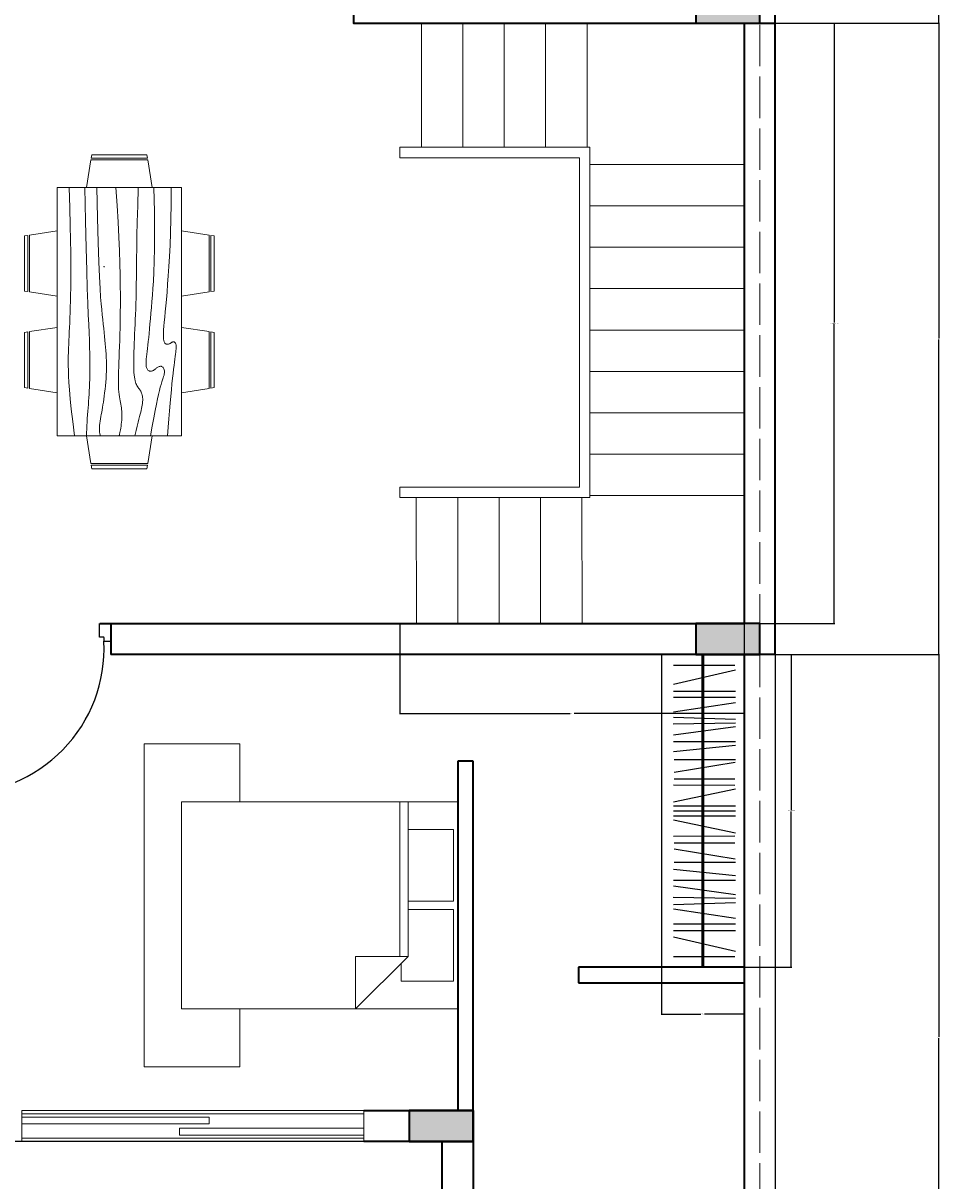
# Model space of a CAD drawing. Units: inches. Extents: x 2711 to 4246, y 540 to 1583.
# Tile 3 of 7: x 3086 to 3351, y 894 to 1230. Entities that reach past the tile are written whole.
import ezdxf

# ---------------------------------------------------------------- set-up
doc = ezdxf.new("R2010")
doc.units = ezdxf.units.IN
doc.linetypes.add('ACAD_ISO02W100', pattern=[15, 12, -3])
for name, color, linetype, lineweight in [('A-ANNO-DIMS', 2, 'Continuous', 18), ('A-COLS', 210, 'Continuous', 35), ('A-COLS-PATT', 6, 'Continuous', 13), ('A-FLOR-CASE', 30, 'Continuous', 18), ('A-FLOR-STRS', 4, 'Continuous', 18), ('A-GLAZ', 4, 'Continuous', 18), ('A-WALL', 1, 'Continuous', 35), ('C-PROP-HIDN', 7, 'ACAD_ISO02W100', 13), ('C-PROP-WALL', 7, 'Continuous', 25), ('DOOR', 32, 'Continuous', 25), ('FURN', 30, 'Continuous', 18)]:
    doc.layers.add(name, color=color, linetype=linetype, lineweight=lineweight)
doc.layers.add('DECOR', color=30, linetype='Continuous')
doc.styles.get("Standard").update_dxf_attribs({"font": 'arial.ttf'})
doc.dimstyles.get("Standard").update_dxf_attribs({"dimtxt": 0.18, "dimasz": 0.18, "dimexe": 0.18, "dimexo": 0.0625, "dimgap": 0.09, "dimtad": 0, "dimtih": 1, "dimtoh": 1, "dimdec": 4, "dimzin": 0, "dimdsep": 46, "dimtxsty": 'Standard', "dimcen": 0.09, "dimadec": 0, "dimazin": 0, "dimtfac": 1, "dimtdec": 4, "dimtofl": 0, "dimtmove": 0, "dimatfit": 3, "dimfxl": 1, "dimtolj": 1, "dimtzin": 0, "dimarcsym": 0})

# ---------------------------------------------------------------- blocks, each defined once
blk = doc.blocks.new('DOORS')
at = {"layer": 'DOOR'}
for p, q in [((-0.63, -0.36), (-0.63, -5.61)), ((2.62, -4.36), (2.62, -0.36)), ((44.12, -4.36), (44.12, -0.36)), ((47.37, -0.36), (47.37, -5.61)), ((-0.63, -5.61), (1.37, -5.61)), ((1.37, -5.61), (1.37, -4.36)), ((1.37, -4.36), (2.62, -4.36)), ((1.37, -5.61), (1.37, -49.61)), ((2.37, -49.61), (2.37, -4.36)), ((45.37, -4.36), (44.12, -4.36)), ((47.37, -5.61), (45.37, -5.61)), ((1.37, -49.61), (2.37, -49.61))]:
    blk.add_line(p, q, dxfattribs=at)
for centre, radius, start, end in [((3.41, -7.61), 42.01, 268.5852, 2.7319), ((38.76, -4.99), 6.64, 354.6023, 5.3977)]:
    blk.add_arc(centre, radius, start, end, dxfattribs=at)
blk = doc.blocks.new('WARDROBE')
at = {"layer": 'DECOR'}
for p, q in [((24, 0), (0, 0)), ((0, 0), (0, -90.69)), ((11.75, 0), (11.75, -90.69)), ((11.78, 0), (11.78, -90.69)), ((11.8, 0), (11.8, -90.69)), ((11.83, 0), (11.83, -90.69)), ((11.85, 0), (11.85, -90.69)), ((11.88, 0), (11.88, -90.69)), ((11.92, 0), (11.92, -90.69)), ((11.95, 0), (11.95, -90.69)), ((11.97, 0), (11.97, -90.69)), ((12, 0), (12, -90.69)), ((12.03, 0), (12.03, -90.69)), ((12.06, 0), (12.06, -90.69)), ((12.1, 0), (12.1, -90.69)), ((12.14, 0), (12.14, -90.69)), ((12.17, 0), (12.17, -90.69)), ((12.2, 0), (12.2, -90.69)), ((12.22, 0), (12.22, -90.69)), ((12.25, 0), (12.25, -90.69)), ((12.25, 0), (12.25, -90.69)), ((24, -90.69), (24, 0)), ((3.53, -3.09), (21.27, -3.09)), ((21.48, -4.58), (3.53, -8.75)), ((3.53, -10.65), (21.48, -10.65)), ((21.48, -12.45), (3.53, -12.45)), ((21.48, -14.08), (3.53, -16.79)), ((21.48, -19.96), (3.47, -20.22)), ((3.53, -18.23), (21.48, -18.75)), ((21.49, -21.01), (3.52, -23.46)), ((3.52, -25.25), (21.49, -25.25)), ((21.49, -26.46), (3.52, -28.29)), ((3.74, -30.44), (21.49, -30.44)), ((21.36, -31.31), (3.74, -34.21)), ((3.74, -36.1), (21.29, -36.1)), ((21.29, -37.99), (3.52, -37.93)), ((3.52, -42.71), (21.49, -38.99)), ((3.52, -43.88), (21.49, -43.88)), ((3.52, -45.34), (21.49, -45.34)), ((3.52, -46.81), (21.49, -46.81)), ((3.52, -47.98), (21.49, -51.69)), ((21.29, -52.7), (3.52, -52.76)), ((3.74, -54.59), (21.29, -54.59)), ((21.36, -59.38), (3.74, -56.48)), ((3.74, -60.25), (21.49, -60.25)), ((21.49, -64.22), (3.52, -62.4)), ((3.52, -65.43), (21.49, -65.43)), ((21.48, -70.73), (3.47, -70.47)), ((21.49, -69.68), (3.52, -67.23)), ((3.53, -72.46), (21.48, -71.94)), ((21.48, -76.61), (3.53, -73.9)), ((21.48, -78.24), (3.53, -78.24)), ((3.53, -80.04), (21.48, -80.04)), ((21.48, -86.1), (3.53, -81.94)), ((3.53, -87.59), (21.27, -87.59)), ((0, -90.69), (24, -90.69))]:
    blk.add_line(p, q, dxfattribs=at)
blk = doc.blocks.new('Bed - Queen')
for p, q in [((0, -80.00003), (0, 0)), ((0, 0), (59.99999, 0)), ((59.99999, 0), (59.99999, -80.00003)), ((7.99999, -1.2), (28.79998, -1.2)), ((7.99999, -14.4), (7.99999, -1.2)), ((28.79998, -1.2), (28.79998, -14.4)), ((31.19999, -1.2), (51.99999, -1.2)), ((31.19999, -14.4), (31.19999, -1.2)), ((51.99999, -1.2), (51.99999, -16.4)), ((0, -14.4), (44.8, -14.4)), ((59.99999, -29.6), (44.8, -14.4)), ((44.8, -14.4), (44.8, -29.6)), ((51.99999, -16.4), (46.79936, -16.4)), ((44.8, -16.8), (0, -16.8)), ((44.8, -29.6), (59.99999, -29.6)), ((59.99999, -80.00003), (0, -80.00003))]:
    blk.add_line(p, q)
blk = doc.blocks.new('Dining Set - 36 x 72 in.')
for p, q in [((-22, 27.5), (-22.1562, 26.50042)), ((-22, 27.5), (-6, 27.5)), ((-5.8437, 26.49966), (-6, 27.5)), ((6, 27.5), (5.8438, 26.50042)), ((6, 27.5), (22, 27.5)), ((22.1563, 26.49966), (22, 27.5)), ((-22.2343, 26.00059), (-23.4847, 17.99762)), ((-22.2304, 26), (-5.7608, 26)), ((-5.8416, 26.5), (-22.1534, 26.5)), ((-4.5152, 17.99762), (-5.7655, 25.99926)), ((5.7657, 26.00059), (4.5153, 17.99762)), ((5.7696, 26), (22.2392, 26)), ((22.1584, 26.5), (5.8466, 26.5)), ((23.4848, 17.99762), (22.2345, 25.99926)), ((36, 18), (-36, 18)), ((-36, 18), (-36, -18)), ((36, -18), (36, 18)), ((-45.5, 8), (-44.5004, 8.15617)), ((-45.5, 8), (-45.5, -8)), ((-44.5, -8.15843), (-44.5, 8.15338)), ((-44.0006, 8.23428), (-35.9976, 9.48474)), ((-44, 8.23041), (-44, -8.23915)), ((44.0006, 8.23428), (35.9976, 9.48474)), ((44, 8.23041), (44, -8.23915)), ((44.5, -8.15843), (44.5, 8.15338)), ((45.5, 8), (44.5005, 8.15617)), ((45.5, 8), (45.5, -8)), ((-44.4997, -8.15631), (-45.5, -8)), ((-35.9976, -9.48476), (-43.9993, -8.2345)), ((35.9976, -9.48476), (43.9993, -8.2345)), ((44.4997, -8.15631), (45.5, -8)), ((-36, -18), (36, -18)), ((-22.2343, -26.0006), (-23.4847, -17.99762)), ((-4.5152, -17.99762), (-5.7655, -25.99928)), ((5.7657, -26.0006), (4.5153, -17.99762)), ((23.4848, -17.99762), (22.2345, -25.99928)), ((-22.2304, -26), (-5.7608, -26)), ((-22, -27.5), (-22.1562, -26.50044)), ((-5.8416, -26.5), (-22.1534, -26.5)), ((-5.8437, -26.49967), (-6, -27.5)), ((5.7696, -26), (22.2392, -26)), ((6, -27.5), (5.8438, -26.50044)), ((22.1584, -26.5), (5.8466, -26.5)), ((22.1563, -26.49967), (22, -27.5)), ((-22, -27.5), (-6, -27.5)), ((6, -27.5), (22, -27.5))]:
    blk.add_line(p, q)
for points in [[(-36, 15), (-31.1772, 14.97754), (-26.8079, 14.91406), (-22.8538, 14.81543), (-19.276, 14.6875), (-16.0362, 14.53613), (-13.0957, 14.36718), (-10.4159, 14.18652), (-7.9583, 14), (-5.6904, 13.81315), (-3.6035, 13.63021), (-1.6954, 13.45508), (0.0365, 13.29166), (1.5945, 13.14388), (2.9811, 13.01562), (4.1988, 12.9108), (5.25, 12.83333), (6.1393, 12.78613), (6.8802, 12.76823), (7.4883, 12.77767), (7.9792, 12.8125), (8.3685, 12.87077), (8.6719, 12.95052), (8.9049, 13.0498), (9.0833, 13.16666), (9.2205, 13.29899), (9.3216, 13.44401), (9.3895, 13.59879), (9.4271, 13.76041), (9.4373, 13.92594), (9.4232, 14.09245), (9.3875, 14.257), (9.3333, 14.41666), (9.2638, 14.56917), (9.1836, 14.71484), (9.0975, 14.85465), (9.0104, 14.98958), (8.9272, 15.1206), (8.8529, 15.2487), (8.7922, 15.37483), (8.75, 15.5), (8.7305, 15.62467), (8.7344, 15.74739), (8.7617, 15.86621), (8.8125, 15.97916), (8.8867, 16.08431), (8.9844, 16.17968), (9.1055, 16.26334), (9.25, 16.33333), (9.4189, 16.38802), (9.6172, 16.42708), (9.8506, 16.45052), (10.125, 16.45833), (10.4463, 16.45052), (10.8203, 16.42708), (11.2529, 16.38802), (11.75, 16.33333), (12.3184, 16.26318), (12.9694, 16.17838), (13.7151, 16.07991), (14.5677, 15.96875), (15.5395, 15.84586), (16.6426, 15.71224), (17.8893, 15.56884), (19.2917, 15.41666), (20.859, 15.25667), (22.5879, 15.08984), (24.4721, 14.91715), (26.5052, 14.73958), (28.6809, 14.5581), (30.9929, 14.3737), (33.4347, 14.18733), (36, 14)], [(-36, 10), (-28.9766, 10.14274), (-23.1725, 10.20442), (-18.4241, 10.19775), (-14.5677, 10.13541), (-11.4399, 10.03011), (-8.877, 9.89453), (-6.7154, 9.74137), (-4.7917, 9.58333), (-2.9698, 9.43082), (-1.2246, 9.28515), (0.4415, 9.14534), (2.026, 9.01041), (3.5266, 8.87939), (4.9408, 8.7513), (6.266, 8.62516), (7.5, 8.5), (8.6411, 8.37549), (9.6914, 8.2539), (10.6538, 8.13818), (11.5312, 8.03125), (12.3267, 7.93603), (13.043, 7.85547), (13.6831, 7.79248), (14.25, 7.75), (14.7471, 7.7303), (15.1797, 7.73307), (15.5537, 7.75732), (15.875, 7.80208), (16.1494, 7.86637), (16.3828, 7.94922), (16.5811, 8.04964), (16.75, 8.16666), (16.8944, 8.29915), (17.0143, 8.44531), (17.1089, 8.60319), (17.1771, 8.77083), (17.218, 8.94629), (17.2305, 9.1276), (17.2137, 9.31282), (17.1667, 9.5), (17.0895, 9.6875), (16.987, 9.875), (16.8649, 10.0625), (16.7292, 10.25), (16.5856, 10.4375), (16.4401, 10.625), (16.2985, 10.8125), (16.1667, 11), (16.05, 11.18733), (15.9518, 11.3737), (15.8752, 11.5581), (15.8229, 11.73958), (15.798, 11.91715), (15.8034, 12.08984), (15.842, 12.25667), (15.9167, 12.41666), (16.0295, 12.56836), (16.1784, 12.70833), (16.3605, 12.83268), (16.5729, 12.9375), (16.8127, 13.01888), (17.0768, 13.07291), (17.3625, 13.0957), (17.6667, 13.08333), (17.9894, 13.03312), (18.3418, 12.94726), (18.7382, 12.82918), (19.1927, 12.68229), (19.7195, 12.51001), (20.3327, 12.31575), (21.0465, 12.10294), (21.875, 11.875), (22.8357, 11.63354), (23.959, 11.37304), (25.2786, 11.08618), (26.8282, 10.76562), (28.6414, 10.40405), (30.752, 9.99414), (33.1936, 9.52856), (36, 9)], [(-36, 5.5), (-30.7157, 5.3348), (-26.069, 5.20963), (-21.9946, 5.11767), (-18.4271, 5.05208), (-15.3009, 5.00602), (-12.5508, 4.97265), (-10.1112, 4.94515), (-7.9167, 4.91666), (-5.909, 4.88167), (-4.0586, 4.83984), (-2.3429, 4.79215), (-0.7396, 4.73958), (0.7739, 4.6831), (2.22, 4.6237), (3.6213, 4.56233), (5, 4.5), (6.373, 4.43782), (7.7344, 4.3776), (9.0723, 4.32129), (10.375, 4.27083), (11.6309, 4.22819), (12.8281, 4.19531), (13.9551, 4.17415), (15, 4.16666), (15.954, 4.17448), (16.819, 4.19791), (17.6001, 4.23698), (18.3021, 4.29166), (18.9299, 4.36198), (19.4883, 4.44791), (19.9823, 4.54948), (20.4167, 4.66666), (20.7969, 4.79899), (21.1302, 4.94401), (21.4245, 5.09879), (21.6875, 5.26041), (21.9271, 5.42594), (22.1511, 5.59245), (22.3672, 5.757), (22.5834, 5.91666), (22.8065, 6.06868), (23.0404, 6.21093), (23.2879, 6.34147), (23.5521, 6.45833), (23.8358, 6.55957), (24.142, 6.64323), (24.4735, 6.70735), (24.8334, 6.75), (25.2235, 6.76969), (25.642, 6.76692), (26.0858, 6.74267), (26.5521, 6.69791), (27.0379, 6.63362), (27.5404, 6.55078), (28.0565, 6.45036), (28.5834, 6.33333), (29.1242, 6.19987), (29.7071, 6.04687), (30.3661, 5.87044), (31.1354, 5.66666), (32.0493, 5.43164), (33.142, 5.16146), (34.4475, 4.85221), (36, 4.5)], [(-36, -1), (-30.7915, -0.6591), (-26.0195, -0.38216), (-21.6519, -0.16284), (-17.6563, 0.00521), (-14.0005, 0.12833), (-10.6523, 0.21289), (-7.5796, 0.26522), (-4.75, 0.29166), (-2.134, 0.29793), (0.2878, 0.28711), (2.5317, 0.26163), (4.6146, 0.22396), (6.5529, 0.17651), (8.3633, 0.12174), (10.0623, 0.06209), (11.6667, 0), (13.1899, -0.06201), (14.6341, -0.1211), (15.9982, -0.17432), (17.2813, -0.21875), (18.4823, -0.25147), (19.6003, -0.26953), (20.6343, -0.27002), (21.5834, -0.25), (22.4481, -0.20768), (23.2357, -0.14584), (23.9549, -0.06836), (24.6146, 0.02083), (25.2235, 0.11784), (25.7904, 0.21875), (26.3241, 0.31966), (26.8334, 0.41666), (27.3265, 0.50618), (27.8099, 0.58593), (28.2894, 0.65397), (28.7709, 0.70833), (29.2601, 0.74707), (29.763, 0.76823), (30.2855, 0.76985), (30.8334, 0.75), (31.4088, 0.70784), (31.9994, 0.64713), (32.589, 0.57275), (33.1615, 0.48958), (33.7008, 0.4025), (34.1908, 0.3164), (34.6153, 0.23616), (34.9584, 0.16666), (35.2099, 0.11165), (35.3848, 0.07031), (35.504, 0.04069), (35.5886, 0.02083), (35.6594, 0.00879), (35.7377, 0.0026), (35.8442, 0.00032), (36, 0)], [(-36, -6.5), (-27.1843, -6.31267), (-20.084, -6.1263), (-14.469, -5.9419), (-10.1094, -5.76042), (-6.7752, -5.58285), (-4.2363, -5.41016), (-2.2629, -5.24333), (-0.625, -5.08334), (0.8708, -4.93099), (2.2715, -4.78646), (3.5872, -4.64974), (4.8281, -4.52084), (6.0046, -4.39974), (7.127, -4.28646), (8.2053, -4.18099), (9.25, -4.08334), (10.2705, -3.99382), (11.2734, -3.91407), (12.2647, -3.84603), (13.25, -3.79167), (14.2354, -3.75293), (15.2266, -3.73177), (16.2295, -3.73015), (17.25, -3.75), (18.2912, -3.79248), (19.3451, -3.85547), (20.4009, -3.93604), (21.4479, -4.03125), (22.4754, -4.13819), (23.4727, -4.25391), (24.4289, -4.37549), (25.3334, -4.5), (26.1785, -4.62492), (26.9694, -4.74935), (27.7145, -4.87281), (28.4219, -4.99479), (29.1, -5.11483), (29.7572, -5.23242), (30.4016, -5.34709), (31.0417, -5.45834), (31.6837, -5.56437), (32.3262, -5.65821), (32.9658, -5.73153), (33.599, -5.77604), (34.2224, -5.78345), (34.8327, -5.74545), (35.4264, -5.65373), (36, -5.5)], [(-36, -10), (-26.4022, -9.81299), (-18.4675, -9.62891), (-11.9839, -9.45069), (-6.7396, -9.28125), (-2.5226, -9.12354), (0.8789, -8.98047), (3.6769, -8.85498), (6.0833, -8.75), (8.2767, -8.66765), (10.3021, -8.60677), (12.1712, -8.56543), (13.8958, -8.54167), (15.4876, -8.53353), (16.9583, -8.53907), (18.3197, -8.55632), (19.5834, -8.58334), (20.7616, -8.61841), (21.8685, -8.66081), (22.9188, -8.71004), (23.9271, -8.76563), (24.9081, -8.82707), (25.8763, -8.89388), (26.8465, -8.96558), (27.8334, -9.04167), (28.8474, -9.12118), (29.8828, -9.20117), (30.93, -9.27824), (31.9792, -9.34896), (33.0205, -9.40991), (34.0443, -9.45768), (35.0407, -9.48885), (36, -9.5)], [(-36, -14.5), (-30.0881, -14.33513), (-25.0332, -14.21224), (-20.7312, -14.12647), (-17.0781, -14.07292), (-13.97, -14.04671), (-11.3027, -14.04297), (-8.9724, -14.05681), (-6.875, -14.08334), (-4.9224, -14.11833), (-3.0905, -14.16016), (-1.3709, -14.20785), (0.2448, -14.26042), (1.7647, -14.3169), (3.1973, -14.3763), (4.5507, -14.43767), (5.8333, -14.5), (7.0554, -14.5621), (8.235, -14.62175), (9.3922, -14.67652), (10.5469, -14.72396), (11.7192, -14.76164), (12.929, -14.78711), (14.1965, -14.79794), (15.5417, -14.79167), (16.9933, -14.76424), (18.6152, -14.70508), (20.4804, -14.60197), (22.6615, -14.44271), (25.2312, -14.21509), (28.2624, -13.9069), (31.8277, -13.50594), (36, -13)]]:
    blk.add_lwpolyline(points)
blk = doc.blocks.new('STAIR-RETURN')
for p, q in [((6.2, 174.01), (6.2, 138.01)), ((18.2, 174.01), (18.2, 138.01)), ((30.2, 174.01), (30.2, 138.01)), ((42.2, 174.01), (42.2, 138.01)), ((54.2, 174.01), (54.2, 138.01)), ((55.04, 138.01), (0, 138.01)), ((0, 138.01), (0, 135.01)), ((55.04, 133.05), (55.04, 138.01)), ((52.04, 135.01), (0, 135.01)), ((52.04, 39.5), (52.04, 135.01)), ((99.72, 133.05), (55.04, 133.05)), ((55.04, 37.05), (55.04, 133.05)), ((99.72, 121.05), (55.04, 121.05)), ((99.72, 109.05), (55.04, 109.05)), ((99.72, 97.05), (55.04, 97.05)), ((99.72, 85.05), (55.04, 85.05)), ((99.72, 73.05), (55.04, 73.05)), ((99.72, 61.05), (55.04, 61.05)), ((99.72, 49.05), (55.04, 49.05)), ((0, 36.5), (0, 39.5)), ((0, 39.5), (52.04, 39.5)), ((99.72, 37.05), (55.04, 37.05)), ((55.04, 36.5), (55.04, 37.05)), ((0, 36.5), (52.73, 36.5)), ((4.73, 36.5), (4.74, 0)), ((16.73, 36.5), (16.74, 0)), ((28.73, 36.5), (28.74, 0)), ((40.73, 36.5), (40.74, 0)), ((52.73, 36.5), (52.74, 0)), ((52.73, 36.5), (55.04, 36.5))]:
    blk.add_line(p, q)
blk = doc.blocks.new('WIN-SLIDER-W03')
for p, q in [((0, 9), (0, 0)), ((99.07, 9), (0, 9)), ((0, 8.03), (99.07, 8.03)), ((0, 7.05), (54.2, 7.05)), ((54.2, 7.05), (54.2, 5.05)), ((99.07, 9), (99.07, 0)), ((54.2, 5.05), (0, 5.05)), ((45.64, 1.82), (45.64, 3.82)), ((45.64, 3.82), (99.07, 3.82)), ((0, 0.97), (99.07, 0.97)), ((99.07, 1.82), (45.64, 1.82)), ((0, 0), (99.07, 0))]:
    blk.add_line(p, q)
blk = doc.blocks.new('BED-BASE-QUEEN')
for p, q in [((27.64, 93.59), (0, 93.59)), ((0, 93.59), (0, 46.79)), ((27.64, 76.79), (27.64, 93.59)), ((0, 0), (0, 46.79)), ((27.64, 16.79), (27.64, 0)), ((27.64, 0), (0, 0))]:
    blk.add_line(p, q)
blk = doc.blocks.new('*D74')
at = {"layer": 'A-ANNO-DIMS', "color": 0, "lineweight": -2, "transparency": 16777216}
for p, q in [((3294.56, 1046.95), (3308.28, 1046.95)), ((3308.1, 1046.77), (3308.1, 1001.79)), ((3308.1, 956.44), (3308.1, 1001.42)), ((3294.56, 956.26), (3308.28, 956.26))]:
    blk.add_line(p, q, dxfattribs=at)
at = {"layer": 'A-ANNO-DIMS', "color": 0, "transparency": 16777216}
for points in [[(3308.07, 1046.77), (3308.13, 1046.77), (3308.1, 1046.95)], [(3308.07, 956.44), (3308.13, 956.44), (3308.1, 956.26)]]:
    blk.add_solid(points, dxfattribs=at)
at = {"layer": 'Defpoints', "color": 0, "transparency": 16777216}
for p in [(3294.5, 1046.95), (3308.1, 1046.95), (3294.5, 956.26)]:
    blk.add_point(p, dxfattribs=at)
at = {"layer": 'A-ANNO-DIMS', "color": 0, "transparency": 16777216, "insert": (3308.1, 1001.61), "char_height": 0.18, "attachment_point": 5}
blk.add_mtext('\\A1;WARDROBE 91 TYP.', dxfattribs=at)
blk = doc.blocks.new('*D75')
at = {"layer": 'A-ANNO-DIMS', "color": 0, "lineweight": -2, "transparency": 16777216}
for p, q in [((3270.5, 956.2), (3270.5, 942.48)), ((3294.5, 956.2), (3294.5, 942.48)), ((3270.68, 942.66), (3281.97, 942.66)), ((3294.32, 942.66), (3283.03, 942.66))]:
    blk.add_line(p, q, dxfattribs=at)
at = {"layer": 'A-ANNO-DIMS', "color": 0, "transparency": 16777216}
for points in [[(3270.68, 942.69), (3270.68, 942.63), (3270.5, 942.66)], [(3294.32, 942.69), (3294.32, 942.63), (3294.5, 942.66)]]:
    blk.add_solid(points, dxfattribs=at)
at = {"layer": 'Defpoints', "color": 0, "transparency": 16777216}
for p in [(3270.5, 956.26), (3294.5, 956.26), (3294.5, 942.66)]:
    blk.add_point(p, dxfattribs=at)
at = {"layer": 'A-ANNO-DIMS', "color": 0, "transparency": 16777216, "insert": (3282.5, 942.66), "char_height": 0.18, "attachment_point": 5}
blk.add_mtext('\\A1;24 TYP.', dxfattribs=at)
blk = doc.blocks.new('*D82')
at = {"layer": 'A-ANNO-DIMS', "color": 0, "lineweight": -2, "transparency": 16777216}
for p, q in [((3294.56, 1229.95), (3320.78, 1229.95)), ((3320.6, 1229.77), (3320.6, 1143.13)), ((3320.6, 1056.12), (3320.6, 1142.76)), ((3294.56, 1055.94), (3320.78, 1055.94))]:
    blk.add_line(p, q, dxfattribs=at)
at = {"layer": 'A-ANNO-DIMS', "color": 0, "transparency": 16777216}
for points in [[(3320.57, 1229.77), (3320.63, 1229.77), (3320.6, 1229.95)], [(3320.57, 1056.12), (3320.63, 1056.12), (3320.6, 1055.94)]]:
    blk.add_solid(points, dxfattribs=at)
at = {"layer": 'Defpoints', "color": 0, "transparency": 16777216}
for p in [(3294.5, 1229.95), (3320.6, 1229.95), (3294.5, 1055.94)]:
    blk.add_point(p, dxfattribs=at)
at = {"layer": 'A-ANNO-DIMS', "color": 0, "transparency": 16777216, "insert": (3320.6, 1142.95), "char_height": 0.18, "attachment_point": 5}
blk.add_mtext('\\A1;RETURN STAIR 174 TYP.', dxfattribs=at)
blk = doc.blocks.new('*D83')
at = {"layer": 'A-ANNO-DIMS', "color": 0, "lineweight": -2, "transparency": 16777216}
for p, q in [((3194.77, 1055.88), (3194.77, 1029.66)), ((3294.5, 1055.88), (3294.5, 1029.66)), ((3194.95, 1029.84), (3244.05, 1029.84)), ((3294.32, 1029.84), (3245.22, 1029.84))]:
    blk.add_line(p, q, dxfattribs=at)
at = {"layer": 'A-ANNO-DIMS', "color": 0, "transparency": 16777216}
for points in [[(3194.95, 1029.87), (3194.95, 1029.81), (3194.77, 1029.84)], [(3294.32, 1029.87), (3294.32, 1029.81), (3294.5, 1029.84)]]:
    blk.add_solid(points, dxfattribs=at)
at = {"layer": 'Defpoints', "color": 0, "transparency": 16777216}
for p in [(3194.77, 1055.94), (3294.5, 1055.94), (3294.5, 1029.84)]:
    blk.add_point(p, dxfattribs=at)
at = {"layer": 'A-ANNO-DIMS', "color": 0, "transparency": 16777216, "insert": (3244.63, 1029.84), "char_height": 0.18, "attachment_point": 5}
blk.add_mtext('\\A1;100 TYP.', dxfattribs=at)
blk = doc.blocks.new('*D99')
at = {"layer": 'A-ANNO-DIMS', "color": 0, "lineweight": -2, "transparency": 16777216}
for p, q in [((3299.06, 1046.94), (3351.05, 1046.94)), ((3350.87, 1046.76), (3350.87, 936.03)), ((3350.87, 824.93), (3350.87, 935.67)), ((3299.06, 824.75), (3351.05, 824.75))]:
    blk.add_line(p, q, dxfattribs=at)
at = {"layer": 'A-ANNO-DIMS', "color": 0, "transparency": 16777216}
for points in [[(3350.84, 1046.76), (3350.9, 1046.76), (3350.87, 1046.94)], [(3350.84, 824.93), (3350.9, 824.93), (3350.87, 824.75)]]:
    blk.add_solid(points, dxfattribs=at)
at = {"layer": 'Defpoints', "color": 0, "transparency": 16777216}
for p in [(3299, 1046.94), (3350.87, 1046.94), (3299, 824.75)]:
    blk.add_point(p, dxfattribs=at)
at = {"layer": 'A-ANNO-DIMS', "color": 0, "transparency": 16777216, "insert": (3350.87, 935.85), "char_height": 0.18, "attachment_point": 5}
blk.add_mtext('\\A1;222.2', dxfattribs=at)
blk = doc.blocks.new('*D100')
at = {"layer": 'A-ANNO-DIMS', "color": 0, "lineweight": -2, "transparency": 16777216}
for p, q in [((3299.06, 1229.95), (3351.05, 1229.95)), ((3350.87, 1229.77), (3350.87, 1138.63)), ((3350.87, 1047.12), (3350.87, 1138.26)), ((3299.06, 1046.94), (3351.05, 1046.94))]:
    blk.add_line(p, q, dxfattribs=at)
at = {"layer": 'A-ANNO-DIMS', "color": 0, "transparency": 16777216}
for points in [[(3350.84, 1229.77), (3350.9, 1229.77), (3350.87, 1229.95)], [(3350.84, 1047.12), (3350.9, 1047.12), (3350.87, 1046.94)]]:
    blk.add_solid(points, dxfattribs=at)
at = {"layer": 'Defpoints', "color": 0, "transparency": 16777216}
for p in [(3299, 1229.95), (3350.87, 1229.95), (3299, 1046.94)]:
    blk.add_point(p, dxfattribs=at)
at = {"layer": 'A-ANNO-DIMS', "color": 0, "transparency": 16777216, "insert": (3350.87, 1138.45), "char_height": 0.18, "attachment_point": 5}
blk.add_mtext('\\A1;183', dxfattribs=at)
blk = doc.blocks.new('*D101')
at = {"layer": 'A-ANNO-DIMS', "color": 0, "lineweight": -2, "transparency": 16777216}
for p, q in [((3209.06, 1289.95), (3351.05, 1289.95)), ((3350.87, 1289.77), (3350.87, 1260.13)), ((3350.87, 1230.13), (3350.87, 1259.77)), ((3299.06, 1229.95), (3351.05, 1229.95))]:
    blk.add_line(p, q, dxfattribs=at)
at = {"layer": 'A-ANNO-DIMS', "color": 0, "transparency": 16777216}
for points in [[(3350.84, 1289.77), (3350.9, 1289.77), (3350.87, 1289.95)], [(3350.84, 1230.13), (3350.9, 1230.13), (3350.87, 1229.95)]]:
    blk.add_solid(points, dxfattribs=at)
at = {"layer": 'Defpoints', "color": 0, "transparency": 16777216}
for p in [(3209, 1289.95), (3350.87, 1289.95), (3299, 1229.95)]:
    blk.add_point(p, dxfattribs=at)
at = {"layer": 'A-ANNO-DIMS', "color": 0, "transparency": 16777216, "insert": (3350.87, 1259.95), "char_height": 0.18, "attachment_point": 5}
blk.add_mtext('\\A1;60', dxfattribs=at)
blk = doc.blocks.new('*D104')
at = {"layer": 'A-ANNO-DIMS', "color": 0, "lineweight": -2, "transparency": 16777216}
for p, q in [((3215.96, 905.77), (2715.94, 905.77)), ((2716.12, 905.59), (2716.12, 865.45)), ((2716.12, 824.95), (2716.12, 865.09)), ((3215.96, 824.77), (2715.94, 824.77))]:
    blk.add_line(p, q, dxfattribs=at)
at = {"layer": 'A-ANNO-DIMS', "color": 0, "transparency": 16777216}
for points in [[(2716.09, 905.59), (2716.15, 905.59), (2716.12, 905.77)], [(2716.09, 824.95), (2716.15, 824.95), (2716.12, 824.77)]]:
    blk.add_solid(points, dxfattribs=at)
at = {"layer": 'Defpoints', "color": 0, "transparency": 16777216}
for p in [(3216.02, 905.77), (2716.12, 824.77), (3216.02, 824.77)]:
    blk.add_point(p, dxfattribs=at)
at = {"layer": 'A-ANNO-DIMS', "color": 0, "transparency": 16777216, "insert": (2716.12, 865.27), "char_height": 0.18, "attachment_point": 5}
blk.add_mtext('\\A1;81', dxfattribs=at)
blk = doc.blocks.new('*D126')
at = {"layer": 'A-ANNO-DIMS', "color": 0, "lineweight": -2, "transparency": 16777216}
for p, q in [((2915.15, 1159.36), (2987.69, 1159.36)), ((3108.98, 1159.36), (3109.16, 1159.36)), ((3109.07, 1159.27), (3109.07, 1159.45))]:
    blk.add_line(p, q, dxfattribs=at)
at = {"layer": 'A-ANNO-DIMS', "color": 0, "transparency": 16777216}
blk.add_solid([(2987.69, 1159.39), (2987.69, 1159.33), (2987.87, 1159.36)], dxfattribs=at)
at = {"layer": 'Defpoints', "color": 0, "transparency": 16777216}
for p in [(2987.87, 1159.36), (3109.07, 1159.36)]:
    blk.add_point(p, dxfattribs=at)
at = {"layer": 'A-ANNO-DIMS', "color": 0, "transparency": 16777216, "insert": (2914.48, 1159.36), "char_height": 0.18, "attachment_point": 5}
blk.add_mtext('\\A1;3X R121.2', dxfattribs=at)

msp = doc.modelspace()

# ---------------------------------------------------------------- hatches: boundary and pattern name
at = {"layer": 'A-COLS-PATT'}
h = msp.add_hatch(color=256, dxfattribs=at)
h.dxf.hatch_style = 1
h.paths.add_polyline_path([(2767.9955, 1384.9055), (2776.9955, 1384.9055), (2776.9955, 1403.4493), (2767.9955, 1403.4493)])
h.paths.add_polyline_path([(3065.5392, 1394.4493), (3065.5392, 1403.4493), (3046.9955, 1403.4493), (3046.9955, 1394.4493)])
h.paths.add_polyline_path([(3298.9955, 1394.4493), (3298.9955, 1403.4493), (3280.4517, 1403.4493), (3280.4517, 1394.4493)])
h.paths.add_polyline_path([(2767.8485, 1230.0438), (2776.8485, 1230.0353), (2776.8485, 1248.5791), (2767.8485, 1248.5791)])
h.paths.add_polyline_path([(2871.9955, 1229.9493), (2871.9955, 1238.9493), (2863.4422, 1238.9493), (2863.4422, 1229.9531), (2867.4955, 1229.9493)])
h.paths.add_polyline_path([(3055.9955, 1229.9493), (3055.9955, 1238.9493), (3037.4517, 1238.9493), (3037.4517, 1229.9493)])
h.paths.add_polyline_path([(3298.9955, 1229.9493), (3298.9955, 1238.9493), (3280.4517, 1238.9493), (3280.4517, 1229.9493)])
h.paths.add_polyline_path([(2776.8485, 1056.0394), (2767.8485, 1056.0394), (2767.8485, 1037.4957), (2776.8485, 1037.4957)])
h.paths.add_polyline_path([(2973.0214, 1041.7894), (2973.0214, 1037.4957), (2982.0148, 1037.4957), (2982.0148, 1056.0394), (2973.0148, 1056.0394), (2973.0148, 1052.2894), (2973.0214, 1052.2894), (2973.0214, 1047.0394)])
h.paths.add_polyline_path([(3063.0214, 1037.4957), (3063.0214, 1056.0394), (3054.0214, 1056.0394), (3054.0214, 1037.4957)])
h.paths.add_polyline_path([(3294.4955, 1046.9493), (3298.9955, 1046.9493), (3298.9955, 1055.9413), (3280.4517, 1055.9413), (3280.4517, 1046.9493)])
h.paths.add_polyline_path([(2982.0214, 924.0394), (2973.0214, 924.0394), (2973.0214, 905.4957), (2982.0214, 905.4957)])
h.paths.add_polyline_path([(3054.0214, 905.4957), (3063.0214, 905.4957), (3063.0214, 924.0394), (3054.0214, 924.0394)])
h.paths.add_polyline_path([(3216.0214, 905.7675), (3216.0214, 914.7675), (3197.4776, 914.7675), (3197.4776, 905.7675)])
h.paths.add_polyline_path([(2776.8485, 842.8947), (2776.8485, 861.4385), (2767.8485, 861.4385), (2767.8485, 842.8947)])
h.paths.add_polyline_path([(3294.4955, 824.7675), (3298.9955, 824.7498), (3298.9955, 833.7498), (3280.4517, 833.7498), (3280.4517, 824.7675)])
h.paths.add_polyline_path([(2793.6045, 587.4493), (2793.6045, 599.3563), (2767.9955, 599.3563), (2767.9955, 587.4493)])
h.paths.add_polyline_path([(2922.1577, 587.4493), (2922.1577, 596.4493), (2913.6045, 596.4493), (2913.6045, 587.4493)])
h.paths.add_polyline_path([(2995.7668, 587.4493), (2995.7668, 599.3563), (2970.1577, 599.3563), (2970.1577, 587.4493)])

# ---------------------------------------------------------------- linework, layer by layer
at = {"layer": 'A-COLS'}
for points in [[(3298.9955, 1238.9493), (3280.4517, 1238.9493), (3280.4517, 1229.9493), (3298.9955, 1229.9493)], [(3298.9955, 1055.9413), (3280.4517, 1055.9413), (3280.4517, 1046.9413), (3298.9955, 1046.9413)], [(3216.0214, 914.7675), (3197.4776, 914.7675), (3197.4776, 905.7675), (3216.0214, 905.7675)]]:
    msp.add_lwpolyline(points, close=True, dxfattribs=at)
at = {"layer": 'A-WALL'}
for p, q in [((3303.4955, 1229.9493), (3303.4955, 1403.4493)), ((3294.4955, 1229.9493), (3294.4955, 1055.9413)), ((3294.4955, 1229.9493), (3294.4955, 1055.9493)), ((3298.9955, 1229.9493), (3303.4955, 1229.9493)), ((3303.4955, 1046.9493), (3303.4955, 1229.9493)), ((3107.7714, 1055.9209), (3111.0214, 1055.9209)), ((3111.0214, 1055.9209), (3294.4955, 1055.9493)), ((3111.0214, 1055.9209), (3111.0214, 1046.9493)), ((3303.4955, 1046.9493), (3111.0214, 1046.9493)), ((3294.4955, 1046.9493), (3294.4955, 833.7498)), ((3216.0214, 1016.0126), (3211.5214, 1016.0126)), ((3211.5214, 1016.0126), (3211.5214, 914.7675)), ((3216.0214, 914.7675), (3216.0214, 1016.0126)), ((3294.4955, 956.2612), (3246.4955, 956.2612)), ((3246.4955, 956.2612), (3246.4955, 951.7612)), ((3246.4955, 951.7612), (3294.4955, 951.7612)), ((3184.3136, 914.7675), (3216.0214, 914.7675)), ((3216.0214, 914.7675), (3216.0214, 905.7675)), ((3216.0214, 905.7675), (3184.3136, 905.7675)), ((3207.0214, 824.7675), (3207.0214, 905.7675)), ((3216.0214, 905.7675), (3216.0214, 833.7675))]:
    msp.add_line(p, q, dxfattribs=at)
msp.add_lwpolyline([(3294.4955, 1238.9493), (3213.4955, 1238.9493), (3181.2888, 1238.9493), (3181.2888, 1229.9493), (3213.4955, 1229.9493), (3294.4955, 1229.9493)], dxfattribs=at)
at = {"layer": 'C-PROP-HIDN'}
msp.add_line((3298.9955, 587.4493), (3298.9955, 1530.4493), dxfattribs=at)
at = {"layer": 'C-PROP-WALL'}
msp.add_line((3303.4955, 1530.4493), (3303.4955, 587.4493), dxfattribs=at)

# ---------------------------------------------------------------- block references
at = {"layer": 'A-FLOR-CASE'}
msp.add_blockref('WARDROBE', (3270.4955, 1046.9493), dxfattribs=at)
at = {"layer": 'A-FLOR-STRS'}
msp.add_blockref('STAIR-RETURN', (3194.774, 1055.942), dxfattribs=at)
at = {"layer": 'A-GLAZ'}
msp.add_blockref('WIN-SLIDER-W03', (3085.247, 905.768), dxfattribs=at)
at = {"layer": 'DOOR'}
msp.add_blockref('DOORS', (3063.6484, 1056.283), dxfattribs=at)
at = {"layer": 'FURN', "rotation": 270}
for name, p in [('Dining Set - 36 x 72 in.', (3113.4661, 1146.2792)), ('Bed - Queen', (3211.5214, 1004.1855))]:
    msp.add_blockref(name, p, dxfattribs=at)
at = {"layer": 'FURN'}
msp.add_blockref('BED-BASE-QUEEN', (3120.6919, 927.3912), dxfattribs=at)

# ---------------------------------------------------------------- dimensions: what is measured, and where the dimension line sits
at = {"layer": 'A-ANNO-DIMS'}
for base, p1, p2, override, picture, middle in [((3350.8725, 1289.9493), (3298.9955, 1229.9493), (3208.9955, 1289.9493), {"dimdec": 0, "dimlfac": 1, "dimrnd": 0, "dimzin": 0, "dimdsep": 46, "dimlunit": 2}, '*D101', (3350.8725, 1259.9493)), ((3350.8725, 1229.9493), (3298.9955, 1046.9413), (3298.9955, 1229.9493), {"dimdec": 0, "dimlfac": 1, "dimrnd": 0, "dimzin": 0, "dimdsep": 46, "dimlunit": 2}, '*D100', (3350.8725, 1138.4453)), ((3350.8725, 1046.9413), (3298.9955, 824.7498), (3298.9955, 1046.9413), {"dimdec": 1, "dimlfac": 1, "dimrnd": 0, "dimzin": 0, "dimdsep": 46, "dimlunit": 2}, '*D99', (3350.8725, 935.8456)), ((2716.1185, 824.7675), (3216.0214, 905.7675), (3216.0214, 824.7675), {"dimdec": 0, "dimlfac": 1, "dimrnd": 0, "dimzin": 0, "dimdsep": 46, "dimlunit": 2}, '*D104', (2716.1185, 865.2675))]:
    dim = msp.add_linear_dim(base=base, p1=p1, p2=p2, angle=90, dimstyle='Standard', override=override, dxfattribs=at)
    dim.commit()
    dim.dimension.update_dxf_attribs({"geometry": picture, "text_midpoint": middle})
for base, p1, p2, text, picture, middle in [((3320.5966, 1229.9493), (3294.4955, 1055.942), (3294.4955, 1229.9493), 'RETURN STAIR <> TYP.', '*D82', (3320.5966, 1142.9456)), ((3308.0987, 1046.9493), (3294.4955, 956.2612), (3294.4955, 1046.9493), 'WARDROBE <> TYP.', '*D74', (3308.0987, 1001.6053))]:
    dim = msp.add_linear_dim(base=base, p1=p1, p2=p2, angle=90, text=text, dimstyle='Standard', override={"dimdec": 0, "dimlfac": 1, "dimrnd": 0, "dimzin": 0, "dimdsep": 46, "dimlunit": 2}, dxfattribs=at)
    dim.commit()
    dim.dimension.update_dxf_attribs({"geometry": picture, "text_midpoint": middle})
dim = msp.add_radius_dim(center=(3109.0685, 1159.3638), mpoint=(2987.8717, 1159.364), text='3X <>', dimstyle='Standard', override={"dimdec": 1, "dimlfac": 1, "dimrnd": 0, "dimzin": 0, "dimdsep": 46, "dimlunit": 2}, dxfattribs=at)
dim.commit()
dim.dimension.update_dxf_attribs({"geometry": '*D126', "text_midpoint": (2915.1537, 1159.3641), "dimtype": 164})
for base, p1, p2, picture, middle in [((3294.4955, 1029.8409), (3194.7744, 1055.942), (3294.4955, 1055.942), '*D83', (3244.635, 1029.8409)), ((3294.4955, 942.658), (3270.4955, 956.2612), (3294.4955, 956.2612), '*D75', (3282.4955, 942.658))]:
    dim = msp.add_linear_dim(base=base, p1=p1, p2=p2, text='<> TYP.', dimstyle='Standard', override={"dimdec": 0, "dimlfac": 1, "dimrnd": 0, "dimzin": 0, "dimdsep": 46, "dimlunit": 2}, dxfattribs=at)
    dim.commit()
    dim.dimension.update_dxf_attribs({"geometry": picture, "text_midpoint": middle})

doc.saveas('drawing.dxf')
